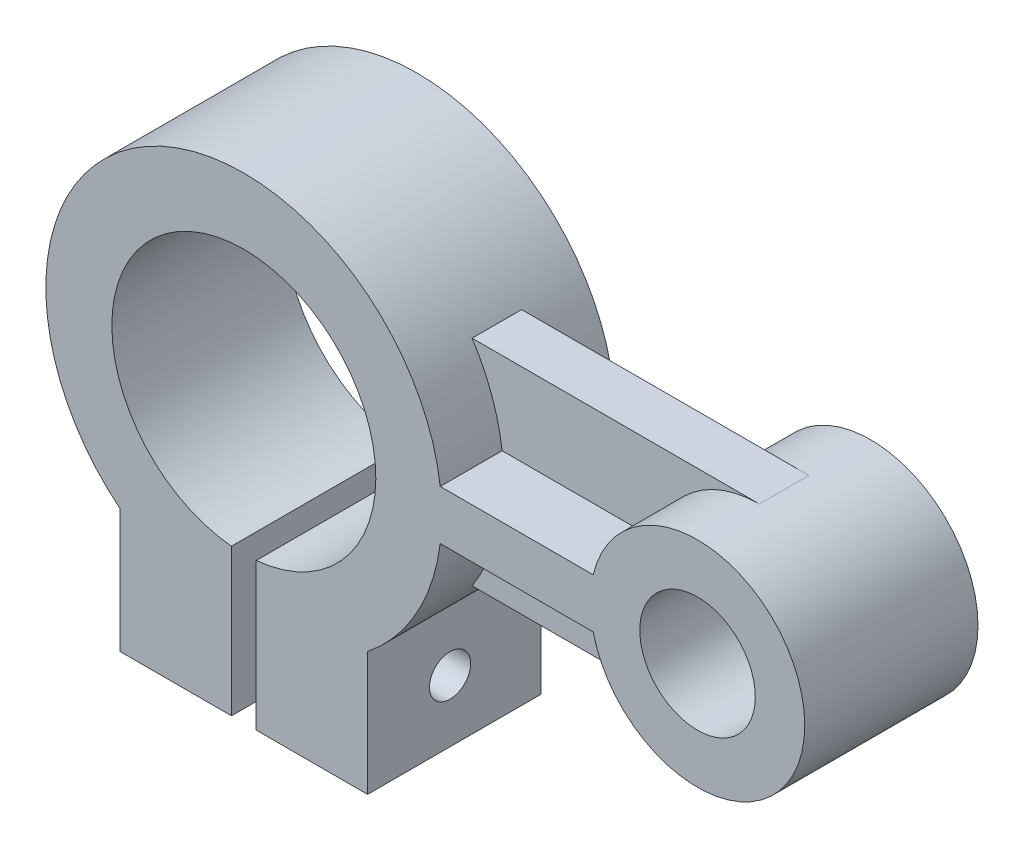
ISO-10303-21;
HEADER;
FILE_DESCRIPTION(('STEP AP214'),'2;1');
FILE_NAME('part.step','',(''),(''),'','','');
FILE_SCHEMA(('AUTOMOTIVE_DESIGN { 1 0 10303 214 1 1 1 1 }'));
ENDSEC;
DATA;
#1=APPLICATION_CONTEXT('core data for automotive mechanical design processes');
#2=APPLICATION_PROTOCOL_DEFINITION('international standard','automotive_design',2000,#1);
#3=PRODUCT_CONTEXT('',#1,'mechanical');
#4=PRODUCT('Part','Part','',(#3));
#5=PRODUCT_RELATED_PRODUCT_CATEGORY('part','',(#4));
#6=PRODUCT_DEFINITION_FORMATION('','',#4);
#7=PRODUCT_DEFINITION_CONTEXT('part definition',#1,'design');
#8=PRODUCT_DEFINITION('design','',#6,#7);
#9=PRODUCT_DEFINITION_SHAPE('','',#8);
#10=(LENGTH_UNIT() NAMED_UNIT(*) SI_UNIT(.MILLI.,.METRE.));
#11=(NAMED_UNIT(*) PLANE_ANGLE_UNIT() SI_UNIT($,.RADIAN.));
#12=(NAMED_UNIT(*) SI_UNIT($,.STERADIAN.) SOLID_ANGLE_UNIT());
#13=UNCERTAINTY_MEASURE_WITH_UNIT(LENGTH_MEASURE(1.E-05),#10,'distance_accuracy_value','');
#14=(GEOMETRIC_REPRESENTATION_CONTEXT(3) GLOBAL_UNCERTAINTY_ASSIGNED_CONTEXT((#13)) GLOBAL_UNIT_ASSIGNED_CONTEXT((#10,
#11,#12)) REPRESENTATION_CONTEXT('',''));
#15=CARTESIAN_POINT('',(0.,0.,0.));
#16=DIRECTION('',(0.,0.,1.));
#17=DIRECTION('',(1.,0.,0.));
#18=AXIS2_PLACEMENT_3D('',#15,#16,#17);
#19=CARTESIAN_POINT('',(40.3197860938899,-6.,-2.));
#20=DIRECTION('',(0.,-1.,0.));
#21=DIRECTION('',(0.,0.,-1.));
#22=AXIS2_PLACEMENT_3D('',#19,#20,#21);
#23=PLANE('',#22);
#24=DIRECTION('',(0.,0.,1.));
#25=VECTOR('',#24,1.);
#26=CARTESIAN_POINT('',(84.7017787186529,-6.,-2.));
#27=LINE('',#26,#25);
#28=CARTESIAN_POINT('',(84.7017787186529,-6.,-2.));
#29=VERTEX_POINT('',#28);
#30=CARTESIAN_POINT('',(84.7017787186529,-6.,13.));
#31=VERTEX_POINT('',#30);
#32=EDGE_CURVE('E257',#29,#31,#27,.T.);
#33=ORIENTED_EDGE('',*,*,#32,.T.);
#34=DIRECTION('',(-1.,0.,0.));
#35=VECTOR('',#34,1.);
#36=CARTESIAN_POINT('',(40.3197860938899,-6.,13.));
#37=LINE('',#36,#35);
#38=CARTESIAN_POINT('',(47.6235235991626,-6.,13.));
#39=VERTEX_POINT('',#38);
#40=EDGE_CURVE('E65',#31,#39,#37,.T.);
#41=ORIENTED_EDGE('',*,*,#40,.T.);
#42=DIRECTION('',(0.,0.,1.));
#43=VECTOR('',#42,1.);
#44=CARTESIAN_POINT('',(47.6235235991626,-6.,-2.));
#45=LINE('',#44,#43);
#46=CARTESIAN_POINT('',(47.6235235991626,-6.,-2.));
#47=VERTEX_POINT('',#46);
#48=EDGE_CURVE('E204',#39,#47,#45,.F.);
#49=ORIENTED_EDGE('',*,*,#48,.T.);
#50=DIRECTION('',(1.,0.,0.));
#51=VECTOR('',#50,1.);
#52=CARTESIAN_POINT('',(40.3197860938899,-6.,-2.));
#53=LINE('',#52,#51);
#54=EDGE_CURVE('E245',#47,#29,#53,.T.);
#55=ORIENTED_EDGE('',*,*,#54,.T.);
#56=EDGE_LOOP('',(#33,#41,#49,#55));
#57=FACE_BOUND('',#56,.T.);
#58=ADVANCED_FACE('F50',(#57),#23,.T.);
#59=CARTESIAN_POINT('',(40.3197860938899,6.,-2.));
#60=DIRECTION('',(0.,1.,0.));
#61=DIRECTION('',(0.,0.,1.));
#62=AXIS2_PLACEMENT_3D('',#59,#60,#61);
#63=PLANE('',#62);
#64=DIRECTION('',(0.,0.,1.));
#65=VECTOR('',#64,1.);
#66=CARTESIAN_POINT('',(84.7017787186529,6.,-2.));
#67=LINE('',#66,#65);
#68=CARTESIAN_POINT('',(84.7017787186529,6.,25.));
#69=VERTEX_POINT('',#68);
#70=CARTESIAN_POINT('',(84.7017787186529,6.,40.));
#71=VERTEX_POINT('',#70);
#72=EDGE_CURVE('E259',#69,#71,#67,.T.);
#73=ORIENTED_EDGE('',*,*,#72,.F.);
#74=DIRECTION('',(-1.,0.,0.));
#75=VECTOR('',#74,1.);
#76=CARTESIAN_POINT('',(40.3197860938899,6.,25.));
#77=LINE('',#76,#75);
#78=CARTESIAN_POINT('',(47.6235235991626,6.,25.));
#79=VERTEX_POINT('',#78);
#80=EDGE_CURVE('E68',#69,#79,#77,.T.);
#81=ORIENTED_EDGE('',*,*,#80,.T.);
#82=DIRECTION('',(0.,0.,1.));
#83=VECTOR('',#82,1.);
#84=CARTESIAN_POINT('',(47.6235235991626,6.,-2.));
#85=LINE('',#84,#83);
#86=CARTESIAN_POINT('',(47.6235235991626,6.,40.));
#87=VERTEX_POINT('',#86);
#88=EDGE_CURVE('E266',#79,#87,#85,.T.);
#89=ORIENTED_EDGE('',*,*,#88,.T.);
#90=DIRECTION('',(-1.,0.,0.));
#91=VECTOR('',#90,1.);
#92=CARTESIAN_POINT('',(40.3197860938899,6.,40.));
#93=LINE('',#92,#91);
#94=EDGE_CURVE('E240',#71,#87,#93,.T.);
#95=ORIENTED_EDGE('',*,*,#94,.F.);
#96=EDGE_LOOP('',(#73,#81,#89,#95));
#97=FACE_BOUND('',#96,.T.);
#98=ADVANCED_FACE('F418',(#97),#63,.T.);
#99=CARTESIAN_POINT('',(0.,0.,-2.));
#100=DIRECTION('',(0.,0.,1.));
#101=DIRECTION('',(1.,0.,0.));
#102=AXIS2_PLACEMENT_3D('',#99,#100,#101);
#103=CYLINDRICAL_SURFACE('',#102,48.);
#104=CARTESIAN_POINT('',(0.,0.,25.));
#105=DIRECTION('',(0.,0.,-1.));
#106=DIRECTION('',(-1.,0.,0.));
#107=AXIS2_PLACEMENT_3D('',#104,#105,#106);
#108=CIRCLE('',#107,48.);
#109=CARTESIAN_POINT('',(40.348482003664,26.,25.));
#110=VERTEX_POINT('',#109);
#111=EDGE_CURVE('E225',#79,#110,#108,.F.);
#112=ORIENTED_EDGE('',*,*,#111,.T.);
#113=DIRECTION('',(0.,0.,1.));
#114=VECTOR('',#113,1.);
#115=CARTESIAN_POINT('',(40.348482003664,26.,-2.));
#116=LINE('',#115,#114);
#117=CARTESIAN_POINT('',(40.348482003664,26.,13.));
#118=VERTEX_POINT('',#117);
#119=EDGE_CURVE('E232',#118,#110,#116,.T.);
#120=ORIENTED_EDGE('',*,*,#119,.F.);
#121=CARTESIAN_POINT('',(0.,0.,13.));
#122=DIRECTION('',(0.,0.,-1.));
#123=DIRECTION('',(-1.,0.,0.));
#124=AXIS2_PLACEMENT_3D('',#121,#122,#123);
#125=CIRCLE('',#124,48.);
#126=CARTESIAN_POINT('',(47.6235235991626,6.,13.));
#127=VERTEX_POINT('',#126);
#128=EDGE_CURVE('E227',#127,#118,#125,.F.);
#129=ORIENTED_EDGE('',*,*,#128,.F.);
#130=CARTESIAN_POINT('',(47.6235235991626,6.,-2.));
#131=VERTEX_POINT('',#130);
#132=EDGE_CURVE('E270',#131,#127,#85,.T.);
#133=ORIENTED_EDGE('',*,*,#132,.F.);
#134=CARTESIAN_POINT('',(0.,0.,-2.));
#135=DIRECTION('',(0.,0.,1.));
#136=DIRECTION('',(1.,0.,0.));
#137=AXIS2_PLACEMENT_3D('',#134,#135,#136);
#138=CIRCLE('',#137,48.);
#139=CARTESIAN_POINT('',(-30.,-37.4699879903904,-2.));
#140=VERTEX_POINT('',#139);
#141=EDGE_CURVE('E309',#131,#140,#138,.T.);
#142=ORIENTED_EDGE('',*,*,#141,.T.);
#143=DIRECTION('',(0.,0.,1.));
#144=VECTOR('',#143,1.);
#145=CARTESIAN_POINT('',(-30.,-37.4699879903904,-2.));
#146=LINE('',#145,#144);
#147=CARTESIAN_POINT('',(-30.,-37.4699879903904,40.));
#148=VERTEX_POINT('',#147);
#149=EDGE_CURVE('E344',#140,#148,#146,.T.);
#150=ORIENTED_EDGE('',*,*,#149,.T.);
#151=CARTESIAN_POINT('',(0.,0.,40.));
#152=DIRECTION('',(0.,0.,1.));
#153=DIRECTION('',(1.,0.,0.));
#154=AXIS2_PLACEMENT_3D('',#151,#152,#153);
#155=CIRCLE('',#154,48.);
#156=EDGE_CURVE('E284',#87,#148,#155,.T.);
#157=ORIENTED_EDGE('',*,*,#156,.F.);
#158=ORIENTED_EDGE('',*,*,#88,.F.);
#159=EDGE_LOOP('',(#112,#120,#129,#133,#142,#150,#157,#158));
#160=FACE_BOUND('',#159,.T.);
#161=ADVANCED_FACE('F373',(#160),#103,.T.);
#162=CARTESIAN_POINT('',(30.,0.,-2.));
#163=DIRECTION('',(1.,0.,0.));
#164=DIRECTION('',(0.,1.,0.));
#165=AXIS2_PLACEMENT_3D('',#162,#163,#164);
#166=PLANE('',#165);
#167=DIRECTION('',(0.,0.,1.));
#168=VECTOR('',#167,1.);
#169=CARTESIAN_POINT('',(30.,-37.4699879903904,-2.));
#170=LINE('',#169,#168);
#171=CARTESIAN_POINT('',(30.,-37.4699879903904,-2.));
#172=VERTEX_POINT('',#171);
#173=CARTESIAN_POINT('',(30.,-37.4699879903904,40.));
#174=VERTEX_POINT('',#173);
#175=EDGE_CURVE('E328',#172,#174,#170,.T.);
#176=ORIENTED_EDGE('',*,*,#175,.T.);
#177=DIRECTION('',(0.,1.,0.));
#178=VECTOR('',#177,1.);
#179=CARTESIAN_POINT('',(30.,0.,40.));
#180=LINE('',#179,#178);
#181=CARTESIAN_POINT('',(30.,-67.4699879903904,40.));
#182=VERTEX_POINT('',#181);
#183=EDGE_CURVE('E285',#182,#174,#180,.T.);
#184=ORIENTED_EDGE('',*,*,#183,.F.);
#185=DIRECTION('',(0.,0.,1.));
#186=VECTOR('',#185,1.);
#187=CARTESIAN_POINT('',(30.,-67.4699879903904,-2.));
#188=LINE('',#187,#186);
#189=CARTESIAN_POINT('',(30.,-67.4699879903904,-2.));
#190=VERTEX_POINT('',#189);
#191=EDGE_CURVE('E329',#190,#182,#188,.T.);
#192=ORIENTED_EDGE('',*,*,#191,.F.);
#193=DIRECTION('',(0.,1.,0.));
#194=VECTOR('',#193,1.);
#195=CARTESIAN_POINT('',(30.,0.,-2.));
#196=LINE('',#195,#194);
#197=EDGE_CURVE('E307',#190,#172,#196,.T.);
#198=ORIENTED_EDGE('',*,*,#197,.T.);
#199=EDGE_LOOP('',(#176,#184,#192,#198));
#200=FACE_BOUND('',#199,.T.);
#201=CARTESIAN_POINT('',(30.,-52.4699879903904,20.));
#202=DIRECTION('',(1.,0.,0.));
#203=DIRECTION('',(0.,1.,0.));
#204=AXIS2_PLACEMENT_3D('',#201,#202,#203);
#205=CIRCLE('',#204,5.);
#206=CARTESIAN_POINT('',(30.,-47.4699879903904,20.));
#207=VERTEX_POINT('',#206);
#208=EDGE_CURVE('E276',#207,#207,#205,.T.);
#209=ORIENTED_EDGE('',*,*,#208,.F.);
#210=EDGE_LOOP('',(#209));
#211=FACE_BOUND('',#210,.T.);
#212=ADVANCED_FACE('F47',(#200,#211),#166,.T.);
#213=CARTESIAN_POINT('',(0.,-67.4699879903904,-2.));
#214=DIRECTION('',(0.,-1.,0.));
#215=DIRECTION('',(0.,0.,-1.));
#216=AXIS2_PLACEMENT_3D('',#213,#214,#215);
#217=PLANE('',#216);
#218=DIRECTION('',(1.,0.,0.));
#219=VECTOR('',#218,1.);
#220=CARTESIAN_POINT('',(0.,-67.4699879903904,40.));
#221=LINE('',#220,#219);
#222=CARTESIAN_POINT('',(2.99999999999991,-67.4699879903904,40.));
#223=VERTEX_POINT('',#222);
#224=EDGE_CURVE('E301',#223,#182,#221,.T.);
#225=ORIENTED_EDGE('',*,*,#224,.F.);
#226=DIRECTION('',(0.,0.,1.));
#227=VECTOR('',#226,1.);
#228=CARTESIAN_POINT('',(2.99999999999991,-67.4699879903904,-2.));
#229=LINE('',#228,#227);
#230=CARTESIAN_POINT('',(2.99999999999991,-67.4699879903904,-2.));
#231=VERTEX_POINT('',#230);
#232=EDGE_CURVE('E335',#231,#223,#229,.T.);
#233=ORIENTED_EDGE('',*,*,#232,.F.);
#234=DIRECTION('',(1.,0.,0.));
#235=VECTOR('',#234,1.);
#236=CARTESIAN_POINT('',(0.,-67.4699879903904,-2.));
#237=LINE('',#236,#235);
#238=EDGE_CURVE('E326',#231,#190,#237,.T.);
#239=ORIENTED_EDGE('',*,*,#238,.T.);
#240=ORIENTED_EDGE('',*,*,#191,.T.);
#241=EDGE_LOOP('',(#225,#233,#239,#240));
#242=FACE_BOUND('',#241,.T.);
#243=ADVANCED_FACE('F405',(#242),#217,.T.);
#244=CARTESIAN_POINT('',(2.99999999999991,0.,-2.));
#245=DIRECTION('',(-1.,0.,0.));
#246=DIRECTION('',(0.,0.,1.));
#247=AXIS2_PLACEMENT_3D('',#244,#245,#246);
#248=PLANE('',#247);
#249=CARTESIAN_POINT('',(2.99999999999991,-52.4699879903904,20.));
#250=DIRECTION('',(-1.,0.,0.));
#251=DIRECTION('',(0.,0.,1.));
#252=AXIS2_PLACEMENT_3D('',#249,#250,#251);
#253=CIRCLE('',#252,5.);
#254=CARTESIAN_POINT('',(2.99999999999991,-52.4699879903904,25.));
#255=VERTEX_POINT('',#254);
#256=EDGE_CURVE('E277',#255,#255,#253,.T.);
#257=ORIENTED_EDGE('',*,*,#256,.F.);
#258=EDGE_LOOP('',(#257));
#259=FACE_BOUND('',#258,.T.);
#260=ORIENTED_EDGE('',*,*,#232,.T.);
#261=DIRECTION('',(0.,-1.,0.));
#262=VECTOR('',#261,1.);
#263=CARTESIAN_POINT('',(2.99999999999991,0.,40.));
#264=LINE('',#263,#262);
#265=CARTESIAN_POINT('',(2.99999999999994,-31.859064644148,40.));
#266=VERTEX_POINT('',#265);
#267=EDGE_CURVE('E302',#266,#223,#264,.T.);
#268=ORIENTED_EDGE('',*,*,#267,.F.);
#269=DIRECTION('',(0.,0.,1.));
#270=VECTOR('',#269,1.);
#271=CARTESIAN_POINT('',(2.99999999999994,-31.859064644148,-2.));
#272=LINE('',#271,#270);
#273=CARTESIAN_POINT('',(2.99999999999994,-31.859064644148,-2.));
#274=VERTEX_POINT('',#273);
#275=EDGE_CURVE('E331',#274,#266,#272,.T.);
#276=ORIENTED_EDGE('',*,*,#275,.F.);
#277=DIRECTION('',(0.,-1.,0.));
#278=VECTOR('',#277,1.);
#279=CARTESIAN_POINT('',(2.99999999999991,0.,-2.));
#280=LINE('',#279,#278);
#281=EDGE_CURVE('E323',#274,#231,#280,.T.);
#282=ORIENTED_EDGE('',*,*,#281,.T.);
#283=EDGE_LOOP('',(#260,#268,#276,#282));
#284=FACE_BOUND('',#283,.T.);
#285=ADVANCED_FACE('F400',(#259,#284),#248,.T.);
#286=CARTESIAN_POINT('',(0.,0.,-2.));
#287=DIRECTION('',(0.,0.,1.));
#288=DIRECTION('',(1.,0.,0.));
#289=AXIS2_PLACEMENT_3D('',#286,#287,#288);
#290=CYLINDRICAL_SURFACE('',#289,32.);
#291=ORIENTED_EDGE('',*,*,#275,.T.);
#292=CARTESIAN_POINT('',(0.,0.,40.));
#293=DIRECTION('',(0.,0.,1.));
#294=DIRECTION('',(1.,0.,0.));
#295=AXIS2_PLACEMENT_3D('',#292,#293,#294);
#296=CIRCLE('',#295,32.);
#297=CARTESIAN_POINT('',(-3.,-31.859064644148,40.));
#298=VERTEX_POINT('',#297);
#299=EDGE_CURVE('E296',#266,#298,#296,.T.);
#300=ORIENTED_EDGE('',*,*,#299,.T.);
#301=DIRECTION('',(0.,0.,1.));
#302=VECTOR('',#301,1.);
#303=CARTESIAN_POINT('',(-3.,-31.859064644148,-2.));
#304=LINE('',#303,#302);
#305=CARTESIAN_POINT('',(-3.,-31.859064644148,-2.));
#306=VERTEX_POINT('',#305);
#307=EDGE_CURVE('E338',#306,#298,#304,.T.);
#308=ORIENTED_EDGE('',*,*,#307,.F.);
#309=CARTESIAN_POINT('',(0.,0.,-2.));
#310=DIRECTION('',(0.,0.,1.));
#311=DIRECTION('',(1.,0.,0.));
#312=AXIS2_PLACEMENT_3D('',#309,#310,#311);
#313=CIRCLE('',#312,32.);
#314=EDGE_CURVE('E321',#274,#306,#313,.T.);
#315=ORIENTED_EDGE('',*,*,#314,.F.);
#316=EDGE_LOOP('',(#291,#300,#308,#315));
#317=FACE_BOUND('',#316,.T.);
#318=ADVANCED_FACE('F391',(#317),#290,.F.);
#319=CARTESIAN_POINT('',(-2.99999999999982,0.,-2.));
#320=DIRECTION('',(-1.,0.,0.));
#321=DIRECTION('',(0.,-1.,0.));
#322=AXIS2_PLACEMENT_3D('',#319,#320,#321);
#323=PLANE('',#322);
#324=CARTESIAN_POINT('',(-3.00000000000011,-52.4699879903904,20.));
#325=DIRECTION('',(-1.,0.,0.));
#326=DIRECTION('',(0.,-1.,0.));
#327=AXIS2_PLACEMENT_3D('',#324,#325,#326);
#328=CIRCLE('',#327,5.);
#329=CARTESIAN_POINT('',(-3.00000000000014,-57.4699879903904,20.));
#330=VERTEX_POINT('',#329);
#331=EDGE_CURVE('E272',#330,#330,#328,.T.);
#332=ORIENTED_EDGE('',*,*,#331,.T.);
#333=EDGE_LOOP('',(#332));
#334=FACE_BOUND('',#333,.T.);
#335=DIRECTION('',(0.,-1.,0.));
#336=VECTOR('',#335,1.);
#337=CARTESIAN_POINT('',(-2.99999999999982,0.,40.));
#338=LINE('',#337,#336);
#339=CARTESIAN_POINT('',(-3.00000000000009,-67.4699879903904,40.));
#340=VERTEX_POINT('',#339);
#341=EDGE_CURVE('E293',#298,#340,#338,.T.);
#342=ORIENTED_EDGE('',*,*,#341,.T.);
#343=DIRECTION('',(0.,0.,1.));
#344=VECTOR('',#343,1.);
#345=CARTESIAN_POINT('',(-3.00000000000009,-67.4699879903904,-2.));
#346=LINE('',#345,#344);
#347=CARTESIAN_POINT('',(-3.00000000000009,-67.4699879903904,-2.));
#348=VERTEX_POINT('',#347);
#349=EDGE_CURVE('E336',#348,#340,#346,.T.);
#350=ORIENTED_EDGE('',*,*,#349,.F.);
#351=DIRECTION('',(0.,-1.,0.));
#352=VECTOR('',#351,1.);
#353=CARTESIAN_POINT('',(-2.99999999999982,0.,-2.));
#354=LINE('',#353,#352);
#355=EDGE_CURVE('E317',#306,#348,#354,.T.);
#356=ORIENTED_EDGE('',*,*,#355,.F.);
#357=ORIENTED_EDGE('',*,*,#307,.T.);
#358=EDGE_LOOP('',(#342,#350,#356,#357));
#359=FACE_BOUND('',#358,.T.);
#360=ADVANCED_FACE('F386',(#334,#359),#323,.F.);
#361=CARTESIAN_POINT('',(0.,-67.4699879903904,-2.));
#362=DIRECTION('',(0.,-1.,0.));
#363=DIRECTION('',(0.,0.,-1.));
#364=AXIS2_PLACEMENT_3D('',#361,#362,#363);
#365=PLANE('',#364);
#366=DIRECTION('',(1.,0.,0.));
#367=VECTOR('',#366,1.);
#368=CARTESIAN_POINT('',(0.,-67.4699879903904,40.));
#369=LINE('',#368,#367);
#370=CARTESIAN_POINT('',(-30.,-67.4699879903904,40.));
#371=VERTEX_POINT('',#370);
#372=EDGE_CURVE('E295',#371,#340,#369,.T.);
#373=ORIENTED_EDGE('',*,*,#372,.F.);
#374=DIRECTION('',(0.,0.,1.));
#375=VECTOR('',#374,1.);
#376=CARTESIAN_POINT('',(-30.,-67.4699879903904,-2.));
#377=LINE('',#376,#375);
#378=CARTESIAN_POINT('',(-30.,-67.4699879903904,-2.));
#379=VERTEX_POINT('',#378);
#380=EDGE_CURVE('E339',#379,#371,#377,.T.);
#381=ORIENTED_EDGE('',*,*,#380,.F.);
#382=DIRECTION('',(1.,0.,0.));
#383=VECTOR('',#382,1.);
#384=CARTESIAN_POINT('',(0.,-67.4699879903904,-2.));
#385=LINE('',#384,#383);
#386=EDGE_CURVE('E316',#379,#348,#385,.T.);
#387=ORIENTED_EDGE('',*,*,#386,.T.);
#388=ORIENTED_EDGE('',*,*,#349,.T.);
#389=EDGE_LOOP('',(#373,#381,#387,#388));
#390=FACE_BOUND('',#389,.T.);
#391=ADVANCED_FACE('F384',(#390),#365,.T.);
#392=CARTESIAN_POINT('',(-30.,0.,-2.));
#393=DIRECTION('',(-1.,0.,0.));
#394=DIRECTION('',(0.,0.,1.));
#395=AXIS2_PLACEMENT_3D('',#392,#393,#394);
#396=PLANE('',#395);
#397=CARTESIAN_POINT('',(-30.,-52.4699879903904,20.));
#398=DIRECTION('',(-1.,0.,0.));
#399=DIRECTION('',(0.,0.,1.));
#400=AXIS2_PLACEMENT_3D('',#397,#398,#399);
#401=CIRCLE('',#400,5.);
#402=CARTESIAN_POINT('',(-30.,-52.4699879903904,25.));
#403=VERTEX_POINT('',#402);
#404=EDGE_CURVE('E269',#403,#403,#401,.T.);
#405=ORIENTED_EDGE('',*,*,#404,.F.);
#406=EDGE_LOOP('',(#405));
#407=FACE_BOUND('',#406,.T.);
#408=ORIENTED_EDGE('',*,*,#380,.T.);
#409=DIRECTION('',(0.,-1.,0.));
#410=VECTOR('',#409,1.);
#411=CARTESIAN_POINT('',(-30.,0.,40.));
#412=LINE('',#411,#410);
#413=EDGE_CURVE('E286',#148,#371,#412,.T.);
#414=ORIENTED_EDGE('',*,*,#413,.F.);
#415=ORIENTED_EDGE('',*,*,#149,.F.);
#416=DIRECTION('',(0.,-1.,0.));
#417=VECTOR('',#416,1.);
#418=CARTESIAN_POINT('',(-30.,0.,-2.));
#419=LINE('',#418,#417);
#420=EDGE_CURVE('E311',#140,#379,#419,.T.);
#421=ORIENTED_EDGE('',*,*,#420,.T.);
#422=EDGE_LOOP('',(#408,#414,#415,#421));
#423=FACE_BOUND('',#422,.T.);
#424=ADVANCED_FACE('F378',(#407,#423),#396,.T.);
#425=CARTESIAN_POINT('',(0.,0.,25.));
#426=DIRECTION('',(0.,0.,1.));
#427=DIRECTION('',(1.,0.,0.));
#428=AXIS2_PLACEMENT_3D('',#425,#426,#427);
#429=CIRCLE('',#428,48.);
#430=CARTESIAN_POINT('',(47.6235235991626,-6.,25.));
#431=VERTEX_POINT('',#430);
#432=CARTESIAN_POINT('',(40.348482003664,-26.,25.));
#433=VERTEX_POINT('',#432);
#434=EDGE_CURVE('E193',#431,#433,#429,.F.);
#435=ORIENTED_EDGE('',*,*,#434,.F.);
#436=CARTESIAN_POINT('',(47.6235235991626,-6.,40.));
#437=VERTEX_POINT('',#436);
#438=EDGE_CURVE('E263',#437,#431,#45,.F.);
#439=ORIENTED_EDGE('',*,*,#438,.F.);
#440=EDGE_CURVE('E287',#174,#437,#155,.T.);
#441=ORIENTED_EDGE('',*,*,#440,.F.);
#442=ORIENTED_EDGE('',*,*,#175,.F.);
#443=EDGE_CURVE('E313',#172,#47,#138,.T.);
#444=ORIENTED_EDGE('',*,*,#443,.T.);
#445=ORIENTED_EDGE('',*,*,#48,.F.);
#446=CARTESIAN_POINT('',(0.,0.,13.));
#447=DIRECTION('',(0.,0.,1.));
#448=DIRECTION('',(1.,0.,0.));
#449=AXIS2_PLACEMENT_3D('',#446,#447,#448);
#450=CIRCLE('',#449,48.);
#451=CARTESIAN_POINT('',(40.348482003664,-26.,13.));
#452=VERTEX_POINT('',#451);
#453=EDGE_CURVE('E196',#39,#452,#450,.F.);
#454=ORIENTED_EDGE('',*,*,#453,.T.);
#455=DIRECTION('',(0.,0.,1.));
#456=VECTOR('',#455,1.);
#457=CARTESIAN_POINT('',(40.348482003664,-26.,-2.));
#458=LINE('',#457,#456);
#459=EDGE_CURVE('E183',#433,#452,#458,.F.);
#460=ORIENTED_EDGE('',*,*,#459,.F.);
#461=EDGE_LOOP('',(#435,#439,#441,#442,#444,#445,#454,#460));
#462=FACE_BOUND('',#461,.T.);
#463=ADVANCED_FACE('F205',(#462),#103,.T.);
#464=CARTESIAN_POINT('',(0.,0.,-2.));
#465=DIRECTION('',(0.,0.,1.));
#466=DIRECTION('',(1.,0.,0.));
#467=AXIS2_PLACEMENT_3D('',#464,#465,#466);
#468=PLANE('',#467);
#469=ORIENTED_EDGE('',*,*,#141,.F.);
#470=DIRECTION('',(-1.,0.,0.));
#471=VECTOR('',#470,1.);
#472=CARTESIAN_POINT('',(40.3197860938899,6.,-2.));
#473=LINE('',#472,#471);
#474=CARTESIAN_POINT('',(84.7017787186529,6.,-2.));
#475=VERTEX_POINT('',#474);
#476=EDGE_CURVE('E238',#475,#131,#473,.T.);
#477=ORIENTED_EDGE('',*,*,#476,.F.);
#478=CARTESIAN_POINT('',(110.,0.,-2.));
#479=DIRECTION('',(0.,0.,1.));
#480=DIRECTION('',(1.,0.,0.));
#481=AXIS2_PLACEMENT_3D('',#478,#479,#480);
#482=CIRCLE('',#481,26.);
#483=EDGE_CURVE('E244',#29,#475,#482,.T.);
#484=ORIENTED_EDGE('',*,*,#483,.F.);
#485=ORIENTED_EDGE('',*,*,#54,.F.);
#486=ORIENTED_EDGE('',*,*,#443,.F.);
#487=ORIENTED_EDGE('',*,*,#197,.F.);
#488=ORIENTED_EDGE('',*,*,#238,.F.);
#489=ORIENTED_EDGE('',*,*,#281,.F.);
#490=ORIENTED_EDGE('',*,*,#314,.T.);
#491=ORIENTED_EDGE('',*,*,#355,.T.);
#492=ORIENTED_EDGE('',*,*,#386,.F.);
#493=ORIENTED_EDGE('',*,*,#420,.F.);
#494=EDGE_LOOP('',(#469,#477,#484,#485,#486,#487,#488,#489,#490,#491,#492,#493));
#495=FACE_BOUND('',#494,.T.);
#496=CARTESIAN_POINT('',(110.,0.,-2.));
#497=DIRECTION('',(0.,0.,1.));
#498=DIRECTION('',(1.,0.,0.));
#499=AXIS2_PLACEMENT_3D('',#496,#497,#498);
#500=CIRCLE('',#499,14.);
#501=CARTESIAN_POINT('',(124.,0.,-2.));
#502=VERTEX_POINT('',#501);
#503=EDGE_CURVE('E231',#502,#502,#500,.T.);
#504=ORIENTED_EDGE('',*,*,#503,.T.);
#505=EDGE_LOOP('',(#504));
#506=FACE_BOUND('',#505,.T.);
#507=ADVANCED_FACE('F368',(#495,#506),#468,.F.);
#508=CARTESIAN_POINT('',(0.,0.,40.));
#509=DIRECTION('',(0.,0.,1.));
#510=DIRECTION('',(1.,0.,0.));
#511=AXIS2_PLACEMENT_3D('',#508,#509,#510);
#512=PLANE('',#511);
#513=ORIENTED_EDGE('',*,*,#440,.T.);
#514=DIRECTION('',(1.,0.,0.));
#515=VECTOR('',#514,1.);
#516=CARTESIAN_POINT('',(40.3197860938899,-6.,40.));
#517=LINE('',#516,#515);
#518=CARTESIAN_POINT('',(84.7017787186529,-6.,40.));
#519=VERTEX_POINT('',#518);
#520=EDGE_CURVE('E253',#437,#519,#517,.T.);
#521=ORIENTED_EDGE('',*,*,#520,.T.);
#522=CARTESIAN_POINT('',(110.,0.,40.));
#523=DIRECTION('',(0.,0.,1.));
#524=DIRECTION('',(1.,0.,0.));
#525=AXIS2_PLACEMENT_3D('',#522,#523,#524);
#526=CIRCLE('',#525,26.);
#527=EDGE_CURVE('E241',#519,#71,#526,.T.);
#528=ORIENTED_EDGE('',*,*,#527,.T.);
#529=ORIENTED_EDGE('',*,*,#94,.T.);
#530=ORIENTED_EDGE('',*,*,#156,.T.);
#531=ORIENTED_EDGE('',*,*,#413,.T.);
#532=ORIENTED_EDGE('',*,*,#372,.T.);
#533=ORIENTED_EDGE('',*,*,#341,.F.);
#534=ORIENTED_EDGE('',*,*,#299,.F.);
#535=ORIENTED_EDGE('',*,*,#267,.T.);
#536=ORIENTED_EDGE('',*,*,#224,.T.);
#537=ORIENTED_EDGE('',*,*,#183,.T.);
#538=EDGE_LOOP('',(#513,#521,#528,#529,#530,#531,#532,#533,#534,#535,#536,#537));
#539=FACE_BOUND('',#538,.T.);
#540=CARTESIAN_POINT('',(110.,0.,40.));
#541=DIRECTION('',(0.,0.,1.));
#542=DIRECTION('',(1.,0.,0.));
#543=AXIS2_PLACEMENT_3D('',#540,#541,#542);
#544=CIRCLE('',#543,14.);
#545=CARTESIAN_POINT('',(124.,0.,40.));
#546=VERTEX_POINT('',#545);
#547=EDGE_CURVE('E235',#546,#546,#544,.T.);
#548=ORIENTED_EDGE('',*,*,#547,.F.);
#549=EDGE_LOOP('',(#548));
#550=FACE_BOUND('',#549,.T.);
#551=ADVANCED_FACE('F381',(#539,#550),#512,.T.);
#552=CARTESIAN_POINT('',(48.,-52.4699879903904,20.));
#553=DIRECTION('',(-1.,0.,0.));
#554=DIRECTION('',(0.,0.,1.));
#555=AXIS2_PLACEMENT_3D('',#552,#553,#554);
#556=CYLINDRICAL_SURFACE('',#555,5.);
#557=ORIENTED_EDGE('',*,*,#331,.F.);
#558=EDGE_LOOP('',(#557));
#559=FACE_BOUND('',#558,.T.);
#560=ORIENTED_EDGE('',*,*,#404,.T.);
#561=EDGE_LOOP('',(#560));
#562=FACE_BOUND('',#561,.T.);
#563=ADVANCED_FACE('F512',(#559,#562),#556,.F.);
#564=ORIENTED_EDGE('',*,*,#208,.T.);
#565=EDGE_LOOP('',(#564));
#566=FACE_BOUND('',#565,.T.);
#567=ORIENTED_EDGE('',*,*,#256,.T.);
#568=EDGE_LOOP('',(#567));
#569=FACE_BOUND('',#568,.T.);
#570=ADVANCED_FACE('F505',(#566,#569),#556,.F.);
#571=DIRECTION('',(-1.,0.,0.));
#572=VECTOR('',#571,1.);
#573=CARTESIAN_POINT('',(40.3197860938899,6.,13.));
#574=LINE('',#573,#572);
#575=CARTESIAN_POINT('',(84.7017787186529,6.,13.));
#576=VERTEX_POINT('',#575);
#577=EDGE_CURVE('E230',#576,#127,#574,.T.);
#578=ORIENTED_EDGE('',*,*,#577,.F.);
#579=EDGE_CURVE('E258',#475,#576,#67,.T.);
#580=ORIENTED_EDGE('',*,*,#579,.F.);
#581=ORIENTED_EDGE('',*,*,#476,.T.);
#582=ORIENTED_EDGE('',*,*,#132,.T.);
#583=EDGE_LOOP('',(#578,#580,#581,#582));
#584=FACE_BOUND('',#583,.T.);
#585=ADVANCED_FACE('F362',(#584),#63,.T.);
#586=CARTESIAN_POINT('',(110.,0.,-2.));
#587=DIRECTION('',(0.,0.,1.));
#588=DIRECTION('',(1.,0.,0.));
#589=AXIS2_PLACEMENT_3D('',#586,#587,#588);
#590=CYLINDRICAL_SURFACE('',#589,26.);
#591=CARTESIAN_POINT('',(110.,0.,25.));
#592=DIRECTION('',(0.,0.,1.));
#593=DIRECTION('',(1.,0.,0.));
#594=AXIS2_PLACEMENT_3D('',#591,#592,#593);
#595=CIRCLE('',#594,26.);
#596=CARTESIAN_POINT('',(110.,-26.,25.));
#597=VERTEX_POINT('',#596);
#598=CARTESIAN_POINT('',(84.7017787186529,-6.,25.));
#599=VERTEX_POINT('',#598);
#600=EDGE_CURVE('E210',#597,#599,#595,.F.);
#601=ORIENTED_EDGE('',*,*,#600,.F.);
#602=DIRECTION('',(0.,0.,1.));
#603=VECTOR('',#602,1.);
#604=CARTESIAN_POINT('',(110.,-26.,-2.));
#605=LINE('',#604,#603);
#606=CARTESIAN_POINT('',(110.,-26.,13.));
#607=VERTEX_POINT('',#606);
#608=EDGE_CURVE('E11',#597,#607,#605,.F.);
#609=ORIENTED_EDGE('',*,*,#608,.T.);
#610=CARTESIAN_POINT('',(110.,0.,13.));
#611=DIRECTION('',(0.,0.,1.));
#612=DIRECTION('',(1.,0.,0.));
#613=AXIS2_PLACEMENT_3D('',#610,#611,#612);
#614=CIRCLE('',#613,26.);
#615=EDGE_CURVE('E200',#607,#31,#614,.F.);
#616=ORIENTED_EDGE('',*,*,#615,.T.);
#617=ORIENTED_EDGE('',*,*,#32,.F.);
#618=ORIENTED_EDGE('',*,*,#483,.T.);
#619=ORIENTED_EDGE('',*,*,#579,.T.);
#620=CARTESIAN_POINT('',(110.,0.,13.));
#621=DIRECTION('',(0.,0.,-1.));
#622=DIRECTION('',(-1.,0.,0.));
#623=AXIS2_PLACEMENT_3D('',#620,#621,#622);
#624=CIRCLE('',#623,26.);
#625=CARTESIAN_POINT('',(110.,26.,13.));
#626=VERTEX_POINT('',#625);
#627=EDGE_CURVE('E223',#626,#576,#624,.F.);
#628=ORIENTED_EDGE('',*,*,#627,.F.);
#629=DIRECTION('',(0.,0.,1.));
#630=VECTOR('',#629,1.);
#631=CARTESIAN_POINT('',(110.,26.,-2.));
#632=LINE('',#631,#630);
#633=CARTESIAN_POINT('',(110.,26.,25.));
#634=VERTEX_POINT('',#633);
#635=EDGE_CURVE('E54',#634,#626,#632,.F.);
#636=ORIENTED_EDGE('',*,*,#635,.F.);
#637=CARTESIAN_POINT('',(110.,0.,25.));
#638=DIRECTION('',(0.,0.,-1.));
#639=DIRECTION('',(-1.,0.,0.));
#640=AXIS2_PLACEMENT_3D('',#637,#638,#639);
#641=CIRCLE('',#640,26.);
#642=EDGE_CURVE('E220',#634,#69,#641,.F.);
#643=ORIENTED_EDGE('',*,*,#642,.T.);
#644=ORIENTED_EDGE('',*,*,#72,.T.);
#645=ORIENTED_EDGE('',*,*,#527,.F.);
#646=EDGE_CURVE('E250',#599,#519,#27,.T.);
#647=ORIENTED_EDGE('',*,*,#646,.F.);
#648=EDGE_LOOP('',(#601,#609,#616,#617,#618,#619,#628,#636,#643,#644,#645,#647));
#649=FACE_BOUND('',#648,.T.);
#650=ADVANCED_FACE('F359',(#649),#590,.T.);
#651=DIRECTION('',(-1.,0.,0.));
#652=VECTOR('',#651,1.);
#653=CARTESIAN_POINT('',(40.3197860938899,-6.,25.));
#654=LINE('',#653,#652);
#655=EDGE_CURVE('E202',#599,#431,#654,.T.);
#656=ORIENTED_EDGE('',*,*,#655,.F.);
#657=ORIENTED_EDGE('',*,*,#646,.T.);
#658=ORIENTED_EDGE('',*,*,#520,.F.);
#659=ORIENTED_EDGE('',*,*,#438,.T.);
#660=EDGE_LOOP('',(#656,#657,#658,#659));
#661=FACE_BOUND('',#660,.T.);
#662=ADVANCED_FACE('F431',(#661),#23,.T.);
#663=CARTESIAN_POINT('',(110.,0.,-2.));
#664=DIRECTION('',(0.,0.,1.));
#665=DIRECTION('',(1.,0.,0.));
#666=AXIS2_PLACEMENT_3D('',#663,#664,#665);
#667=CYLINDRICAL_SURFACE('',#666,14.);
#668=CARTESIAN_POINT('',(124.,0.,40.));
#669=CARTESIAN_POINT('',(124.,0.,39.5625));
#670=CARTESIAN_POINT('',(124.,0.,39.125));
#671=CARTESIAN_POINT('',(124.,0.,38.25));
#672=CARTESIAN_POINT('',(124.,0.,37.8125));
#673=CARTESIAN_POINT('',(124.,0.,36.9375));
#674=CARTESIAN_POINT('',(124.,0.,36.5));
#675=CARTESIAN_POINT('',(124.,0.,35.625));
#676=CARTESIAN_POINT('',(124.,0.,35.1875));
#677=CARTESIAN_POINT('',(124.,0.,34.3125));
#678=CARTESIAN_POINT('',(124.,0.,33.875));
#679=CARTESIAN_POINT('',(124.,0.,33.));
#680=CARTESIAN_POINT('',(124.,0.,32.5625));
#681=CARTESIAN_POINT('',(124.,0.,31.6875));
#682=CARTESIAN_POINT('',(124.,0.,31.25));
#683=CARTESIAN_POINT('',(124.,0.,30.375));
#684=CARTESIAN_POINT('',(124.,0.,29.9375));
#685=CARTESIAN_POINT('',(124.,0.,29.0625));
#686=CARTESIAN_POINT('',(124.,0.,28.625));
#687=CARTESIAN_POINT('',(124.,0.,27.75));
#688=CARTESIAN_POINT('',(124.,0.,27.3125));
#689=CARTESIAN_POINT('',(124.,0.,26.4375));
#690=CARTESIAN_POINT('',(124.,0.,26.));
#691=CARTESIAN_POINT('',(124.,0.,25.125));
#692=CARTESIAN_POINT('',(124.,0.,24.6875));
#693=CARTESIAN_POINT('',(124.,0.,23.8125));
#694=CARTESIAN_POINT('',(124.,0.,23.375));
#695=CARTESIAN_POINT('',(124.,0.,22.5));
#696=CARTESIAN_POINT('',(124.,0.,22.0625));
#697=CARTESIAN_POINT('',(124.,0.,21.1875));
#698=CARTESIAN_POINT('',(124.,0.,20.75));
#699=CARTESIAN_POINT('',(124.,0.,19.875));
#700=CARTESIAN_POINT('',(124.,0.,19.4375));
#701=CARTESIAN_POINT('',(124.,0.,18.5625));
#702=CARTESIAN_POINT('',(124.,0.,18.125));
#703=CARTESIAN_POINT('',(124.,0.,17.25));
#704=CARTESIAN_POINT('',(124.,0.,16.8125));
#705=CARTESIAN_POINT('',(124.,0.,15.9375));
#706=CARTESIAN_POINT('',(124.,0.,15.5));
#707=CARTESIAN_POINT('',(124.,0.,14.625));
#708=CARTESIAN_POINT('',(124.,0.,14.1875));
#709=CARTESIAN_POINT('',(124.,0.,13.3125));
#710=CARTESIAN_POINT('',(124.,0.,12.875));
#711=CARTESIAN_POINT('',(124.,0.,12.));
#712=CARTESIAN_POINT('',(124.,0.,11.5625));
#713=CARTESIAN_POINT('',(124.,0.,10.6875));
#714=CARTESIAN_POINT('',(124.,0.,10.25));
#715=CARTESIAN_POINT('',(124.,0.,9.375));
#716=CARTESIAN_POINT('',(124.,0.,8.9375));
#717=CARTESIAN_POINT('',(124.,0.,8.0625));
#718=CARTESIAN_POINT('',(124.,0.,7.625));
#719=CARTESIAN_POINT('',(124.,0.,6.75));
#720=CARTESIAN_POINT('',(124.,0.,6.3125));
#721=CARTESIAN_POINT('',(124.,0.,5.4375));
#722=CARTESIAN_POINT('',(124.,0.,5.));
#723=CARTESIAN_POINT('',(124.,0.,4.125));
#724=CARTESIAN_POINT('',(124.,0.,3.6875));
#725=CARTESIAN_POINT('',(124.,0.,2.8125));
#726=CARTESIAN_POINT('',(124.,0.,2.375));
#727=CARTESIAN_POINT('',(124.,0.,1.5));
#728=CARTESIAN_POINT('',(124.,0.,1.0625));
#729=CARTESIAN_POINT('',(124.,0.,0.1875));
#730=CARTESIAN_POINT('',(124.,0.,-0.250000000000001));
#731=CARTESIAN_POINT('',(124.,0.,-1.125));
#732=CARTESIAN_POINT('',(124.,0.,-1.5625));
#733=CARTESIAN_POINT('',(124.,0.,-2.));
#734=B_SPLINE_CURVE_WITH_KNOTS('',3,(#668,#669,#670,#671,#672,#673,#674,#675,#676,#677,#678,
#679,#680,#681,#682,#683,#684,#685,#686,#687,#688,#689,#690,#691,#692,#693,#694,#695,#696,#697,
#698,#699,#700,#701,#702,#703,#704,#705,#706,#707,#708,#709,#710,#711,#712,#713,#714,#715,#716,
#717,#718,#719,#720,#721,#722,#723,#724,#725,#726,#727,#728,#729,#730,#731,#732,#733),
.UNSPECIFIED.,.F.,.F.,(4,2,2,2,2,2,2,2,2,2,2,2,2,2,2,2,2,2,2,2,2,2,2,2,2,2,2,2,2,2,2,2,4),(0.,
1.3125,2.625,3.9375,5.25,6.5625,7.875,9.1875,10.5,11.8125,13.125,14.4375,15.75,17.0625,18.375,
19.6875,21.,22.3125,23.625,24.9375,26.25,27.5625,28.875,30.1875,31.5,32.8125,34.125,35.4375,
36.75,38.0625,39.375,40.6875,42.),.UNSPECIFIED.);
#735=EDGE_CURVE('BSEAM426',#546,#502,#734,.T.);
#736=ORIENTED_EDGE('',*,*,#547,.T.);
#737=ORIENTED_EDGE('',*,*,#503,.F.);
#738=ORIENTED_EDGE('',*,*,#735,.T.);
#739=ORIENTED_EDGE('',*,*,#735,.F.);
#740=EDGE_LOOP('',(#736,#738,#737,#739));
#741=FACE_BOUND('',#740,.T.);
#742=ADVANCED_FACE('F426',(#741),#667,.F.);
#743=CARTESIAN_POINT('',(18.7862402391061,26.,13.));
#744=DIRECTION('',(0.,0.,-1.));
#745=DIRECTION('',(-1.,0.,0.));
#746=AXIS2_PLACEMENT_3D('',#743,#744,#745);
#747=PLANE('',#746);
#748=ORIENTED_EDGE('',*,*,#577,.T.);
#749=ORIENTED_EDGE('',*,*,#128,.T.);
#750=DIRECTION('',(-1.,0.,0.));
#751=VECTOR('',#750,1.);
#752=CARTESIAN_POINT('',(18.7862402391061,26.,13.));
#753=LINE('',#752,#751);
#754=EDGE_CURVE('E212',#118,#626,#753,.F.);
#755=ORIENTED_EDGE('',*,*,#754,.T.);
#756=ORIENTED_EDGE('',*,*,#627,.T.);
#757=EDGE_LOOP('',(#748,#749,#755,#756));
#758=FACE_BOUND('',#757,.T.);
#759=ADVANCED_FACE('F351',(#758),#747,.T.);
#760=CARTESIAN_POINT('',(18.7862402391061,26.,25.));
#761=DIRECTION('',(0.,0.,-1.));
#762=DIRECTION('',(-1.,0.,0.));
#763=AXIS2_PLACEMENT_3D('',#760,#761,#762);
#764=PLANE('',#763);
#765=ORIENTED_EDGE('',*,*,#111,.F.);
#766=ORIENTED_EDGE('',*,*,#80,.F.);
#767=ORIENTED_EDGE('',*,*,#642,.F.);
#768=DIRECTION('',(-1.,0.,0.));
#769=VECTOR('',#768,1.);
#770=CARTESIAN_POINT('',(18.7862402391061,26.,25.));
#771=LINE('',#770,#769);
#772=EDGE_CURVE('E191',#110,#634,#771,.F.);
#773=ORIENTED_EDGE('',*,*,#772,.F.);
#774=EDGE_LOOP('',(#765,#766,#767,#773));
#775=FACE_BOUND('',#774,.T.);
#776=ADVANCED_FACE('F416',(#775),#764,.F.);
#777=CARTESIAN_POINT('',(110.350889359326,26.,19.));
#778=DIRECTION('',(0.,1.,0.));
#779=DIRECTION('',(1.,0.,0.));
#780=AXIS2_PLACEMENT_3D('',#777,#778,#779);
#781=PLANE('',#780);
#782=ORIENTED_EDGE('',*,*,#754,.F.);
#783=ORIENTED_EDGE('',*,*,#119,.T.);
#784=ORIENTED_EDGE('',*,*,#772,.T.);
#785=ORIENTED_EDGE('',*,*,#635,.T.);
#786=EDGE_LOOP('',(#782,#783,#784,#785));
#787=FACE_BOUND('',#786,.T.);
#788=ADVANCED_FACE('F350',(#787),#781,.T.);
#789=CARTESIAN_POINT('',(110.350889359326,-26.,19.));
#790=DIRECTION('',(0.,-1.,0.));
#791=DIRECTION('',(1.,0.,0.));
#792=AXIS2_PLACEMENT_3D('',#789,#790,#791);
#793=PLANE('',#792);
#794=DIRECTION('',(1.,0.,0.));
#795=VECTOR('',#794,1.);
#796=CARTESIAN_POINT('',(30.,-26.,25.));
#797=LINE('',#796,#795);
#798=EDGE_CURVE('E189',#433,#597,#797,.T.);
#799=ORIENTED_EDGE('',*,*,#798,.F.);
#800=ORIENTED_EDGE('',*,*,#459,.T.);
#801=DIRECTION('',(1.,0.,0.));
#802=VECTOR('',#801,1.);
#803=CARTESIAN_POINT('',(30.,-26.,13.));
#804=LINE('',#803,#802);
#805=EDGE_CURVE('E186',#452,#607,#804,.T.);
#806=ORIENTED_EDGE('',*,*,#805,.T.);
#807=ORIENTED_EDGE('',*,*,#608,.F.);
#808=EDGE_LOOP('',(#799,#800,#806,#807));
#809=FACE_BOUND('',#808,.T.);
#810=ADVANCED_FACE('F190',(#809),#793,.T.);
#811=CARTESIAN_POINT('',(30.,-26.,25.));
#812=DIRECTION('',(0.,0.,1.));
#813=DIRECTION('',(1.,0.,0.));
#814=AXIS2_PLACEMENT_3D('',#811,#812,#813);
#815=PLANE('',#814);
#816=ORIENTED_EDGE('',*,*,#655,.T.);
#817=ORIENTED_EDGE('',*,*,#434,.T.);
#818=ORIENTED_EDGE('',*,*,#798,.T.);
#819=ORIENTED_EDGE('',*,*,#600,.T.);
#820=EDGE_LOOP('',(#816,#817,#818,#819));
#821=FACE_BOUND('',#820,.T.);
#822=ADVANCED_FACE('F448',(#821),#815,.T.);
#823=CARTESIAN_POINT('',(30.,-26.,13.));
#824=DIRECTION('',(0.,0.,1.));
#825=DIRECTION('',(1.,0.,0.));
#826=AXIS2_PLACEMENT_3D('',#823,#824,#825);
#827=PLANE('',#826);
#828=ORIENTED_EDGE('',*,*,#453,.F.);
#829=ORIENTED_EDGE('',*,*,#40,.F.);
#830=ORIENTED_EDGE('',*,*,#615,.F.);
#831=ORIENTED_EDGE('',*,*,#805,.F.);
#832=EDGE_LOOP('',(#828,#829,#830,#831));
#833=FACE_BOUND('',#832,.T.);
#834=ADVANCED_FACE('F197',(#833),#827,.F.);
#835=CLOSED_SHELL('',(#58,#98,#161,#212,#243,#285,#318,#360,#391,#424,#463,#507,#551,#563,#570,
#585,#650,#662,#742,#759,#776,#788,#810,#822,#834));
#836=MANIFOLD_SOLID_BREP('B2',#835);
#837=ADVANCED_BREP_SHAPE_REPRESENTATION('',(#18,#836),#14);
#838=SHAPE_DEFINITION_REPRESENTATION(#9,#837);
ENDSEC;
END-ISO-10303-21;
